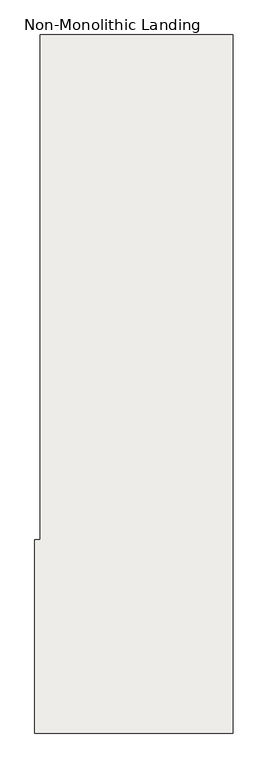
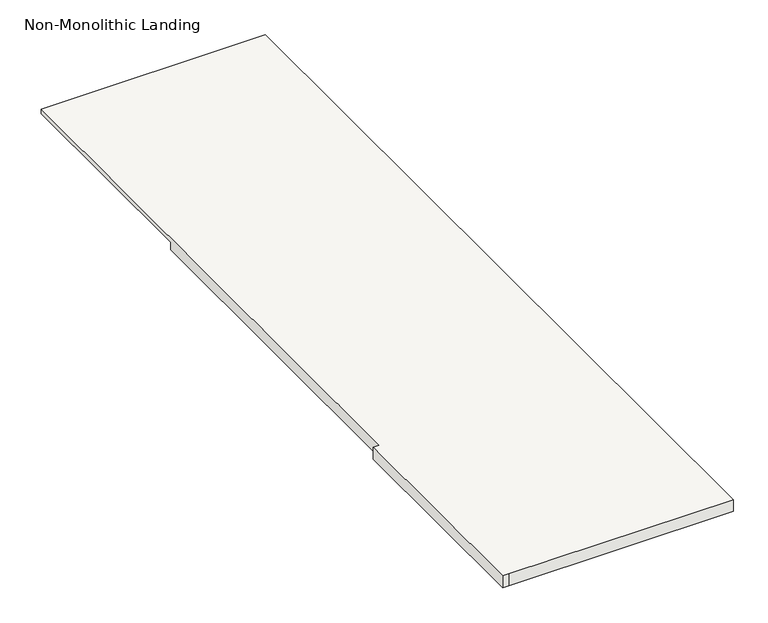
"""IFC4 building model written with IfcOpenShell, lengths in millimetres: slab geometry, Non-Monolithic Landing."""

from ifc_helpers import new_model, si_unit, origin, place, context, project, spatial, faceted_brep, source, transform, mapped, element, save


def non_monolithic_landing_bdf883c6(model_context):
    return source(origin(), model_context, "Body", "Brep", [
        faceted_brep([(-7602.2399968, 11387.7610583, 827.6166667), (-7576.8399968, 11387.7610583, 802.2166667), (-7576.8399968, 10473.3610583, 802.2166667), (-7602.2399968, 10473.3610583, 827.6166667), (-7602.2399968, 8997.8426639, 846.6666667), (-7627.6399968, 8997.8426639, 846.6666667), (-7627.6399968, 8083.4426639, 846.6666667), (-7602.2399968, 8083.4426639, 846.6666667), (-6687.8399968, 8083.4426639, 846.6666667), (-6687.8399968, 11387.7610583, 846.6666667), (-7602.2399968, 11387.7610583, 846.6666667), (-7576.8399968, 10473.3610583, 795.8666667), (-7576.8399968, 11387.7610583, 795.8666667), (-6687.8399968, 11387.7610583, 795.8666667), (-6687.8399968, 8083.4426639, 795.8666667), (-7602.2399968, 8083.4426639, 795.8666667), (-7627.6399968, 8083.4426639, 795.8666667), (-7627.6399968, 8997.8426639, 795.8666667), (-7602.2399968, 8997.8426639, 795.8666667), (-7602.2399968, 10473.3610583, 795.8666667)], [[[0, 1, 2, 3]], [[4, 5, 6, 7, 8, 9, 10]], [[11, 12, 13, 14, 15, 16, 17, 18, 19]], [[12, 11, 2, 1]], [[11, 19, 3, 2]], [[4, 10, 0, 3, 19, 18]], [[5, 4, 18, 17]], [[6, 5, 17, 16]], [[7, 6, 16, 15]], [[8, 7, 15, 14]], [[9, 8, 14, 13]], [[10, 9, 13, 12, 1, 0]]]),
    ])


if __name__ == "__main__":
    model = new_model("IFC4")
    model_context = context("Model", 3, world=origin())
    ifc_project = project(units=[si_unit("LENGTHUNIT", "METRE", prefix="MILLI")], contexts=[model_context])
    site = spatial("IfcSite", under=ifc_project)
    building = spatial("IfcBuilding", under=site)
    placement = place(None, origin())
    non_monolithic_landing_shape = non_monolithic_landing_bdf883c6(model_context)
    element("IfcSlab", 1, ObjectType="Non-Monolithic Landing", at=placement, inside=building, context=model_context, shape_type="MappedRepresentation", body=[
        mapped(non_monolithic_landing_shape, transform((0.0, 0.0, 0.0), x_axis=(1.0, 0.0, 0.0), y_axis=(0.0, 1.0, 0.0), z_axis=(0.0, 0.0, 1.0))),
    ])
    save(model, "model.ifc")
